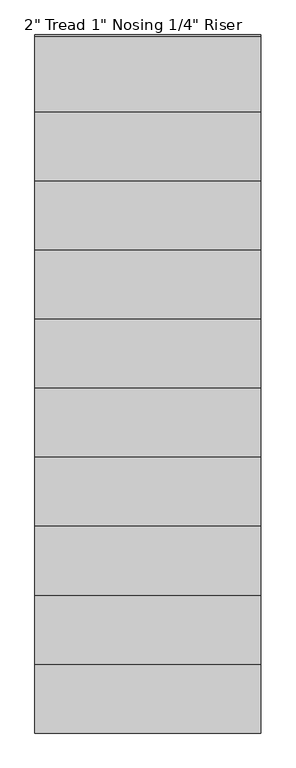
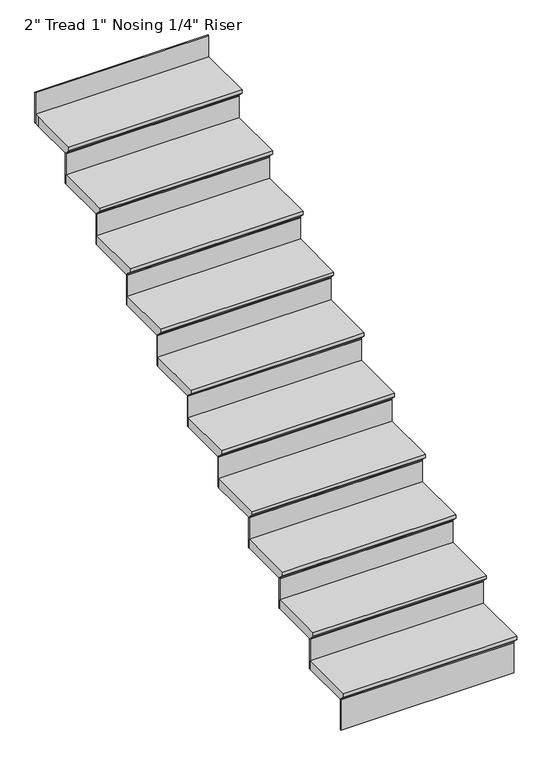
"""IFC4 building model written with IfcOpenShell, lengths in millimetres: stair flight geometry."""

from ifc_helpers import new_model, si_unit, origin, place, context, project, spatial, faceted_brep, source, transform, mapped, element, save


def stair_flight_cee2f43a(model_context):
    return source(origin(), model_context, "Body", "Brep", [
        faceted_brep([(-14022.18283, 4844.1500793, 2182.2833333), (-14022.18283, 4844.1500793, 2201.3333333), (-14936.58283, 4844.1500793, 2201.3333333), (-14936.58283, 4844.1500793, 2182.2833333), (-14022.18283, 4869.5500793, 2156.8833333), (-14936.58283, 4869.5500793, 2156.8833333), (-14022.18283, 5148.9500793, 2201.3333333), (-14936.58283, 5148.9500793, 2201.3333333), (-14936.58283, 4869.5500793, 2150.5333333), (-14936.58283, 5148.9500793, 2150.5333333), (-14022.18283, 5148.9500793, 2150.5333333), (-14022.18283, 4869.5500793, 2150.5333333)], [[[0, 1, 2, 3]], [[4, 0, 3, 5]], [[2, 1, 6, 7]], [[8, 9, 10, 11]], [[2, 7, 9, 8, 5, 3]], [[8, 11, 4, 5]], [[6, 1, 0, 4, 11, 10]], [[7, 6, 10, 9]]]),
        faceted_brep([(-14022.18283, 4869.5500793, 2150.5333333), (-14022.18283, 4869.5500793, 1981.2), (-14022.18283, 4875.9000793, 1981.2), (-14022.18283, 4875.9000793, 2150.5333333), (-14936.58283, 4869.5500793, 2150.5333333), (-14936.58283, 4875.9000793, 2150.5333333), (-14936.58283, 4875.9000793, 1981.2), (-14936.58283, 4869.5500793, 1981.2)], [[[0, 1, 2, 3]], [[4, 5, 6, 7]], [[1, 0, 4, 7]], [[2, 1, 7, 6]], [[3, 2, 6, 5]], [[0, 3, 5, 4]]]),
        faceted_brep([(-14022.18283, 5148.9500793, 2319.8666667), (-14022.18283, 5148.9500793, 2150.5333333), (-14022.18283, 5155.3000793, 2150.5333333), (-14022.18283, 5155.3000793, 2319.8666667), (-14936.58283, 5148.9500793, 2319.8666667), (-14936.58283, 5155.3000793, 2319.8666667), (-14936.58283, 5155.3000793, 2150.5333333), (-14936.58283, 5148.9500793, 2150.5333333)], [[[0, 1, 2, 3]], [[4, 5, 6, 7]], [[1, 0, 4, 7]], [[2, 1, 7, 6]], [[3, 2, 6, 5]], [[0, 3, 5, 4]]]),
        faceted_brep([(-14936.58283, 5123.5500793, 2370.6666667), (-14022.18283, 5123.5500793, 2370.6666667), (-14022.18283, 5428.3500793, 2370.6666667), (-14936.58283, 5428.3500793, 2370.6666667), (-14936.58283, 5148.9500793, 2319.8666667), (-14936.58283, 5428.3500793, 2319.8666667), (-14022.18283, 5428.3500793, 2319.8666667), (-14022.18283, 5148.9500793, 2319.8666667), (-14936.58283, 5148.9500793, 2326.2166667), (-14936.58283, 5123.5500793, 2351.6166667), (-14022.18283, 5148.9500793, 2326.2166667), (-14022.18283, 5123.5500793, 2351.6166667)], [[[0, 1, 2, 3]], [[4, 5, 6, 7]], [[0, 3, 5, 4, 8, 9]], [[4, 7, 10, 8]], [[2, 1, 11, 10, 7, 6]], [[3, 2, 6, 5]], [[11, 1, 0, 9]], [[10, 11, 9, 8]]]),
        faceted_brep([(-14022.18283, 5428.3500793, 2489.2), (-14022.18283, 5428.3500793, 2319.8666667), (-14022.18283, 5434.7000793, 2319.8666667), (-14022.18283, 5434.7000793, 2489.2), (-14936.58283, 5428.3500793, 2489.2), (-14936.58283, 5434.7000793, 2489.2), (-14936.58283, 5434.7000793, 2319.8666667), (-14936.58283, 5428.3500793, 2319.8666667)], [[[0, 1, 2, 3]], [[4, 5, 6, 7]], [[1, 0, 4, 7]], [[2, 1, 7, 6]], [[3, 2, 6, 5]], [[0, 3, 5, 4]]]),
        faceted_brep([(-14936.58283, 5402.9500793, 2540.0), (-14022.18283, 5402.9500793, 2540.0), (-14022.18283, 5707.7500793, 2540.0), (-14936.58283, 5707.7500793, 2540.0), (-14936.58283, 5428.3500793, 2489.2), (-14936.58283, 5707.7500793, 2489.2), (-14022.18283, 5707.7500793, 2489.2), (-14022.18283, 5428.3500793, 2489.2), (-14936.58283, 5428.3500793, 2495.55), (-14936.58283, 5402.9500793, 2520.95), (-14022.18283, 5428.3500793, 2495.55), (-14022.18283, 5402.9500793, 2520.95)], [[[0, 1, 2, 3]], [[4, 5, 6, 7]], [[0, 3, 5, 4, 8, 9]], [[4, 7, 10, 8]], [[2, 1, 11, 10, 7, 6]], [[3, 2, 6, 5]], [[11, 1, 0, 9]], [[10, 11, 9, 8]]]),
        faceted_brep([(-14022.18283, 5707.7500793, 2658.5333333), (-14022.18283, 5707.7500793, 2489.2), (-14022.18283, 5714.1000793, 2489.2), (-14022.18283, 5714.1000793, 2658.5333333), (-14936.58283, 5707.7500793, 2658.5333333), (-14936.58283, 5714.1000793, 2658.5333333), (-14936.58283, 5714.1000793, 2489.2), (-14936.58283, 5707.7500793, 2489.2)], [[[0, 1, 2, 3]], [[4, 5, 6, 7]], [[1, 0, 4, 7]], [[2, 1, 7, 6]], [[3, 2, 6, 5]], [[0, 3, 5, 4]]]),
        faceted_brep([(-14936.58283, 5682.3500793, 2709.3333333), (-14022.18283, 5682.3500793, 2709.3333333), (-14022.18283, 5987.1500793, 2709.3333333), (-14936.58283, 5987.1500793, 2709.3333333), (-14936.58283, 5707.7500793, 2658.5333333), (-14936.58283, 5987.1500793, 2658.5333333), (-14022.18283, 5987.1500793, 2658.5333333), (-14022.18283, 5707.7500793, 2658.5333333), (-14936.58283, 5707.7500793, 2664.8833333), (-14936.58283, 5682.3500793, 2690.2833333), (-14022.18283, 5707.7500793, 2664.8833333), (-14022.18283, 5682.3500793, 2690.2833333)], [[[0, 1, 2, 3]], [[4, 5, 6, 7]], [[0, 3, 5, 4, 8, 9]], [[4, 7, 10, 8]], [[2, 1, 11, 10, 7, 6]], [[3, 2, 6, 5]], [[11, 1, 0, 9]], [[10, 11, 9, 8]]]),
        faceted_brep([(-14022.18283, 5987.1500793, 2827.8666667), (-14022.18283, 5987.1500793, 2658.5333333), (-14022.18283, 5993.5000793, 2658.5333333), (-14022.18283, 5993.5000793, 2827.8666667), (-14936.58283, 5987.1500793, 2827.8666667), (-14936.58283, 5993.5000793, 2827.8666667), (-14936.58283, 5993.5000793, 2658.5333333), (-14936.58283, 5987.1500793, 2658.5333333)], [[[0, 1, 2, 3]], [[4, 5, 6, 7]], [[1, 0, 4, 7]], [[2, 1, 7, 6]], [[3, 2, 6, 5]], [[0, 3, 5, 4]]]),
        faceted_brep([(-14936.58283, 5961.7500793, 2878.6666667), (-14022.18283, 5961.7500793, 2878.6666667), (-14022.18283, 6266.5500793, 2878.6666667), (-14936.58283, 6266.5500793, 2878.6666667), (-14936.58283, 5987.1500793, 2827.8666667), (-14936.58283, 6266.5500793, 2827.8666667), (-14022.18283, 6266.5500793, 2827.8666667), (-14022.18283, 5987.1500793, 2827.8666667), (-14936.58283, 5987.1500793, 2834.2166667), (-14936.58283, 5961.7500793, 2859.6166667), (-14022.18283, 5987.1500793, 2834.2166667), (-14022.18283, 5961.7500793, 2859.6166667)], [[[0, 1, 2, 3]], [[4, 5, 6, 7]], [[0, 3, 5, 4, 8, 9]], [[4, 7, 10, 8]], [[2, 1, 11, 10, 7, 6]], [[3, 2, 6, 5]], [[11, 1, 0, 9]], [[10, 11, 9, 8]]]),
        faceted_brep([(-14022.18283, 6266.5500793, 2997.2), (-14022.18283, 6266.5500793, 2827.8666667), (-14022.18283, 6272.9000793, 2827.8666667), (-14022.18283, 6272.9000793, 2997.2), (-14936.58283, 6266.5500793, 2997.2), (-14936.58283, 6272.9000793, 2997.2), (-14936.58283, 6272.9000793, 2827.8666667), (-14936.58283, 6266.5500793, 2827.8666667)], [[[0, 1, 2, 3]], [[4, 5, 6, 7]], [[1, 0, 4, 7]], [[2, 1, 7, 6]], [[3, 2, 6, 5]], [[0, 3, 5, 4]]]),
        faceted_brep([(-14936.58283, 6241.1500793, 3048.0), (-14022.18283, 6241.1500793, 3048.0), (-14022.18283, 6545.9500793, 3048.0), (-14936.58283, 6545.9500793, 3048.0), (-14936.58283, 6266.5500793, 2997.2), (-14936.58283, 6545.9500793, 2997.2), (-14022.18283, 6545.9500793, 2997.2), (-14022.18283, 6266.5500793, 2997.2), (-14936.58283, 6266.5500793, 3003.55), (-14936.58283, 6241.1500793, 3028.95), (-14022.18283, 6266.5500793, 3003.55), (-14022.18283, 6241.1500793, 3028.95)], [[[0, 1, 2, 3]], [[4, 5, 6, 7]], [[0, 3, 5, 4, 8, 9]], [[4, 7, 10, 8]], [[2, 1, 11, 10, 7, 6]], [[3, 2, 6, 5]], [[11, 1, 0, 9]], [[10, 11, 9, 8]]]),
        faceted_brep([(-14022.18283, 6545.9500793, 3166.5333333), (-14022.18283, 6545.9500793, 2997.2), (-14022.18283, 6552.3000793, 2997.2), (-14022.18283, 6552.3000793, 3166.5333333), (-14936.58283, 6545.9500793, 3166.5333333), (-14936.58283, 6552.3000793, 3166.5333333), (-14936.58283, 6552.3000793, 2997.2), (-14936.58283, 6545.9500793, 2997.2)], [[[0, 1, 2, 3]], [[4, 5, 6, 7]], [[1, 0, 4, 7]], [[2, 1, 7, 6]], [[3, 2, 6, 5]], [[0, 3, 5, 4]]]),
        faceted_brep([(-14936.58283, 6520.5500793, 3217.3333333), (-14022.18283, 6520.5500793, 3217.3333333), (-14022.18283, 6825.3500793, 3217.3333333), (-14936.58283, 6825.3500793, 3217.3333333), (-14936.58283, 6545.9500793, 3166.5333333), (-14936.58283, 6825.3500793, 3166.5333333), (-14022.18283, 6825.3500793, 3166.5333333), (-14022.18283, 6545.9500793, 3166.5333333), (-14936.58283, 6545.9500793, 3172.8833333), (-14936.58283, 6520.5500793, 3198.2833333), (-14022.18283, 6545.9500793, 3172.8833333), (-14022.18283, 6520.5500793, 3198.2833333)], [[[0, 1, 2, 3]], [[4, 5, 6, 7]], [[0, 3, 5, 4, 8, 9]], [[4, 7, 10, 8]], [[2, 1, 11, 10, 7, 6]], [[3, 2, 6, 5]], [[11, 1, 0, 9]], [[10, 11, 9, 8]]]),
        faceted_brep([(-14022.18283, 6825.3500793, 3335.8666667), (-14022.18283, 6825.3500793, 3166.5333333), (-14022.18283, 6831.7000793, 3166.5333333), (-14022.18283, 6831.7000793, 3335.8666667), (-14936.58283, 6825.3500793, 3335.8666667), (-14936.58283, 6831.7000793, 3335.8666667), (-14936.58283, 6831.7000793, 3166.5333333), (-14936.58283, 6825.3500793, 3166.5333333)], [[[0, 1, 2, 3]], [[4, 5, 6, 7]], [[1, 0, 4, 7]], [[2, 1, 7, 6]], [[3, 2, 6, 5]], [[0, 3, 5, 4]]]),
        faceted_brep([(-14936.58283, 6799.9500793, 3386.6666667), (-14022.18283, 6799.9500793, 3386.6666667), (-14022.18283, 7104.7500793, 3386.6666667), (-14936.58283, 7104.7500793, 3386.6666667), (-14936.58283, 6825.3500793, 3335.8666667), (-14936.58283, 7104.7500793, 3335.8666667), (-14022.18283, 7104.7500793, 3335.8666667), (-14022.18283, 6825.3500793, 3335.8666667), (-14936.58283, 6825.3500793, 3342.2166667), (-14936.58283, 6799.9500793, 3367.6166667), (-14022.18283, 6825.3500793, 3342.2166667), (-14022.18283, 6799.9500793, 3367.6166667)], [[[0, 1, 2, 3]], [[4, 5, 6, 7]], [[0, 3, 5, 4, 8, 9]], [[4, 7, 10, 8]], [[2, 1, 11, 10, 7, 6]], [[3, 2, 6, 5]], [[11, 1, 0, 9]], [[10, 11, 9, 8]]]),
        faceted_brep([(-14022.18283, 7104.7500793, 3505.2), (-14022.18283, 7104.7500793, 3335.8666667), (-14022.18283, 7111.1000793, 3335.8666667), (-14022.18283, 7111.1000793, 3505.2), (-14936.58283, 7104.7500793, 3505.2), (-14936.58283, 7111.1000793, 3505.2), (-14936.58283, 7111.1000793, 3335.8666667), (-14936.58283, 7104.7500793, 3335.8666667)], [[[0, 1, 2, 3]], [[4, 5, 6, 7]], [[1, 0, 4, 7]], [[2, 1, 7, 6]], [[3, 2, 6, 5]], [[0, 3, 5, 4]]]),
        faceted_brep([(-14936.58283, 7079.3500793, 3556.0), (-14022.18283, 7079.3500793, 3556.0), (-14022.18283, 7384.1500793, 3556.0), (-14936.58283, 7384.1500793, 3556.0), (-14936.58283, 7104.7500793, 3505.2), (-14936.58283, 7384.1500793, 3505.2), (-14022.18283, 7384.1500793, 3505.2), (-14022.18283, 7104.7500793, 3505.2), (-14936.58283, 7104.7500793, 3511.55), (-14936.58283, 7079.3500793, 3536.95), (-14022.18283, 7104.7500793, 3511.55), (-14022.18283, 7079.3500793, 3536.95)], [[[0, 1, 2, 3]], [[4, 5, 6, 7]], [[0, 3, 5, 4, 8, 9]], [[4, 7, 10, 8]], [[2, 1, 11, 10, 7, 6]], [[3, 2, 6, 5]], [[11, 1, 0, 9]], [[10, 11, 9, 8]]]),
        faceted_brep([(-14022.18283, 7663.5500793, 3843.8666667), (-14022.18283, 7663.5500793, 3674.5333333), (-14022.18283, 7669.9000793, 3674.5333333), (-14022.18283, 7669.9000793, 3843.8666667), (-14936.58283, 7663.5500793, 3843.8666667), (-14936.58283, 7669.9000793, 3843.8666667), (-14936.58283, 7669.9000793, 3674.5333333), (-14936.58283, 7663.5500793, 3674.5333333)], [[[0, 1, 2, 3]], [[4, 5, 6, 7]], [[1, 0, 4, 7]], [[2, 1, 7, 6]], [[3, 2, 6, 5]], [[0, 3, 5, 4]]]),
        faceted_brep([(-14022.18283, 7384.1500793, 3674.5333333), (-14022.18283, 7384.1500793, 3505.2), (-14022.18283, 7390.5000793, 3505.2), (-14022.18283, 7390.5000793, 3674.5333333), (-14936.58283, 7384.1500793, 3674.5333333), (-14936.58283, 7390.5000793, 3674.5333333), (-14936.58283, 7390.5000793, 3505.2), (-14936.58283, 7384.1500793, 3505.2)], [[[0, 1, 2, 3]], [[4, 5, 6, 7]], [[1, 0, 4, 7]], [[2, 1, 7, 6]], [[3, 2, 6, 5]], [[0, 3, 5, 4]]]),
        faceted_brep([(-14936.58283, 7663.5500793, 3725.3333333), (-14936.58283, 7638.1500793, 3725.3333333), (-14936.58283, 7358.7500793, 3725.3333333), (-14022.18283, 7358.7500793, 3725.3333333), (-14022.18283, 7638.1500793, 3725.3333333), (-14022.18283, 7663.5500793, 3725.3333333), (-14936.58283, 7638.1500793, 3674.5333333), (-14936.58283, 7663.5500793, 3674.5333333), (-14022.18283, 7663.5500793, 3674.5333333), (-14022.18283, 7638.1500793, 3674.5333333), (-14022.18283, 7384.1500793, 3674.5333333), (-14936.58283, 7384.1500793, 3674.5333333), (-14936.58283, 7384.1500793, 3680.8833333), (-14936.58283, 7358.7500793, 3706.2833333), (-14022.18283, 7384.1500793, 3680.8833333), (-14022.18283, 7358.7500793, 3706.2833333)], [[[0, 1, 2, 3, 4, 5]], [[6, 7, 8, 9, 10, 11]], [[1, 0, 7, 6]], [[2, 1, 6, 11, 12, 13]], [[11, 10, 14, 12]], [[4, 3, 15, 14, 10, 9]], [[5, 4, 9, 8]], [[0, 5, 8, 7]], [[15, 3, 2, 13]], [[14, 15, 13, 12]]]),
    ])


if __name__ == "__main__":
    model = new_model("IFC4")
    model_context = context("Model", 3, world=origin())
    ifc_project = project(units=[si_unit("LENGTHUNIT", "METRE", prefix="MILLI")], contexts=[model_context])
    site = spatial("IfcSite", under=ifc_project)
    building = spatial("IfcBuilding", under=site)
    placement = place(None, origin())
    stair_flight_shape = stair_flight_cee2f43a(model_context)
    element("IfcStairFlight", 1, ObjectType="2\" Tread 1\" Nosing 1/4\" Riser", at=placement, inside=building, context=model_context, shape_type="MappedRepresentation", body=[
        mapped(stair_flight_shape, transform((0.0, 0.0, 0.0), x_axis=(1.0, 0.0, 0.0), y_axis=(0.0, 1.0, 0.0), z_axis=(0.0, 0.0, 1.0))),
    ])
    save(model, "model.ifc")
